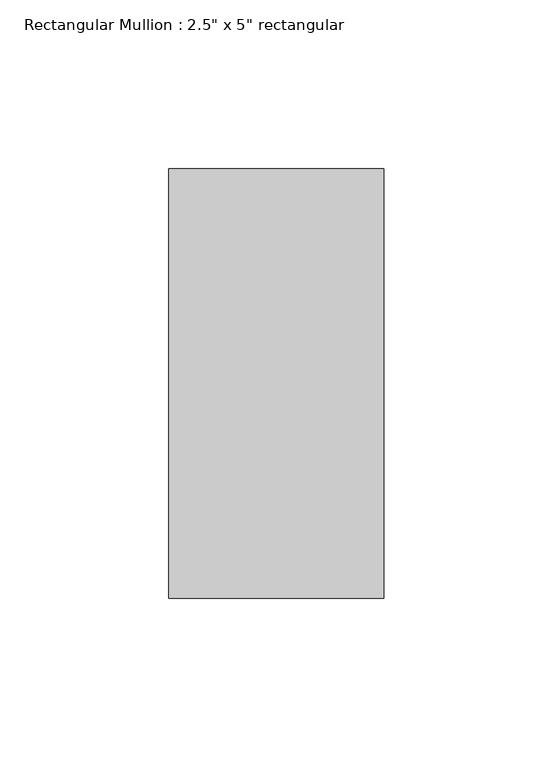
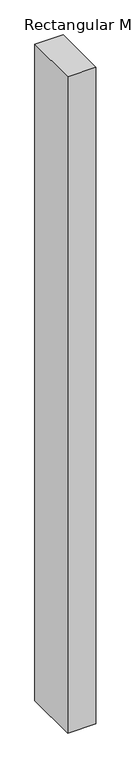
"""IFC4 building model written with IfcOpenShell, lengths in millimetres: member geometry."""

from ifc_helpers import new_model, si_unit, frame, origin, place, context, project, spatial, polyline, outline, extrude, source, transform, mapped, element, save


def member_aafbdc53(model_context):
    return source(origin(), model_context, "Body", "SweptSolid", [
        extrude(outline(polyline([(31.75, 63.5), (31.75, -63.5), (-31.75, -63.5), (-31.75, 63.5), (31.75, 63.5)])), frame((0.0, 0.0, -1555.75), z_axis=(0.0, 0.0, 1.0), x_axis=(1.0, 0.0, 0.0)), (0.0, 0.0, 1.0), 1555.75),
    ])


if __name__ == "__main__":
    model = new_model("IFC4")
    model_context = context("Model", 3, world=origin())
    ifc_project = project(units=[si_unit("LENGTHUNIT", "METRE", prefix="MILLI")], contexts=[model_context])
    site = spatial("IfcSite", under=ifc_project)
    building = spatial("IfcBuilding", under=site)
    placement = place(None, origin())
    member_shape = member_aafbdc53(model_context)
    element("IfcMember", 1, ObjectType="Rectangular Mullion : 2.5\" x 5\" rectangular", at=placement, inside=building, context=model_context, shape_type="MappedRepresentation", body=[
        mapped(member_shape, transform((0.0, 0.0, 0.0), x_axis=(1.0, 0.0, 0.0), y_axis=(0.0, 1.0, 0.0), z_axis=(0.0, 0.0, 1.0))),
    ])
    save(model, "model.ifc")

# Revit data of these elements
# Type "Rectangular Mullion : 2.5\" x 5\" rectangular"
#   built-in parameter 1007304 = 0.416667 (stored number, unit not read)
#   built-in parameter 1007301 = 0.104167 (stored number, unit not read)
#   built-in parameter 1007300 = 0.104167 (stored number, unit not read)
# Element 1 (IfcMember, "Rectangular Mullion : 2.5\" x 5\" rectangular")
#   Materials on its faces: "Aluminum"
# Materials
#   "Aluminum": class "Metal", colour RGB 247 247 247, transparency 0, Description = "Aluminum 6061", Cost = 0
